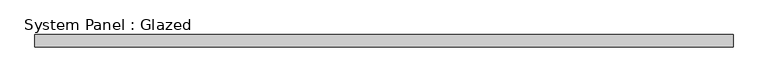
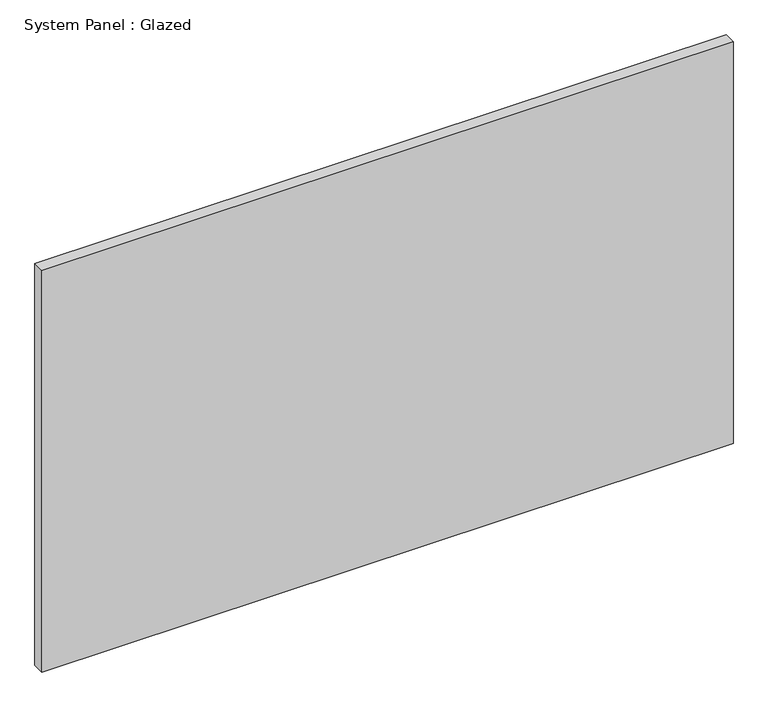
"""IFC4 building model written with IfcOpenShell, lengths in millimetres: plate geometry, System Panel : Glazed."""

from ifc_helpers import new_model, si_unit, origin, origin_with_axes, place, context, project, spatial, polyline, outline, extrude, source, transform, mapped, element, save


def system_panel_glazed_c86d0b30(model_context):
    return source(origin(), model_context, "Body", "SweptSolid", [
        extrude(outline(polyline([(730.25, 19.05), (-730.25, 19.05), (-730.25, 44.45), (730.25, 44.45), (730.25, 19.05)])), origin_with_axes(), (0.0, 0.0, 1.0), 897.5064813),
    ])


if __name__ == "__main__":
    model = new_model("IFC4")
    model_context = context("Model", 3, world=origin())
    ifc_project = project(units=[si_unit("LENGTHUNIT", "METRE", prefix="MILLI")], contexts=[model_context])
    site = spatial("IfcSite", under=ifc_project)
    building = spatial("IfcBuilding", under=site)
    placement = place(None, origin())
    system_panel_glazed_shape = system_panel_glazed_c86d0b30(model_context)
    element("IfcPlate", 1, ObjectType="System Panel : Glazed", at=placement, inside=building, context=model_context, shape_type="MappedRepresentation", body=[
        mapped(system_panel_glazed_shape, transform((0.0, 0.0, 0.0), x_axis=(1.0, 0.0, 0.0), y_axis=(0.0, 1.0, 0.0), z_axis=(0.0, 0.0, 1.0))),
    ])
    save(model, "model.ifc")

# Revit data of these elements
# Type "System Panel : Glazed"
#   Construction Type Id = "GSP4R"
#   Analytic Construction = "1/8 in Pilkington single glazing"
#   Visual Light Transmittance = 0.9
#   Solar Heat Gain Coefficient = 0.86
#   Heat Transfer Coefficient (U) = 1.18115 BTU/(h·ft²·°F)
#   Define Thermal Properties by = 1
# Element 1 (IfcPlate, "System Panel : Glazed")
#   Materials on its faces: "Glass"
# Materials
#   "Glass": class "Glass", colour RGB 0 128 192, transparency 0.75, Description = "Soda Lime Glass", Cost = 0
